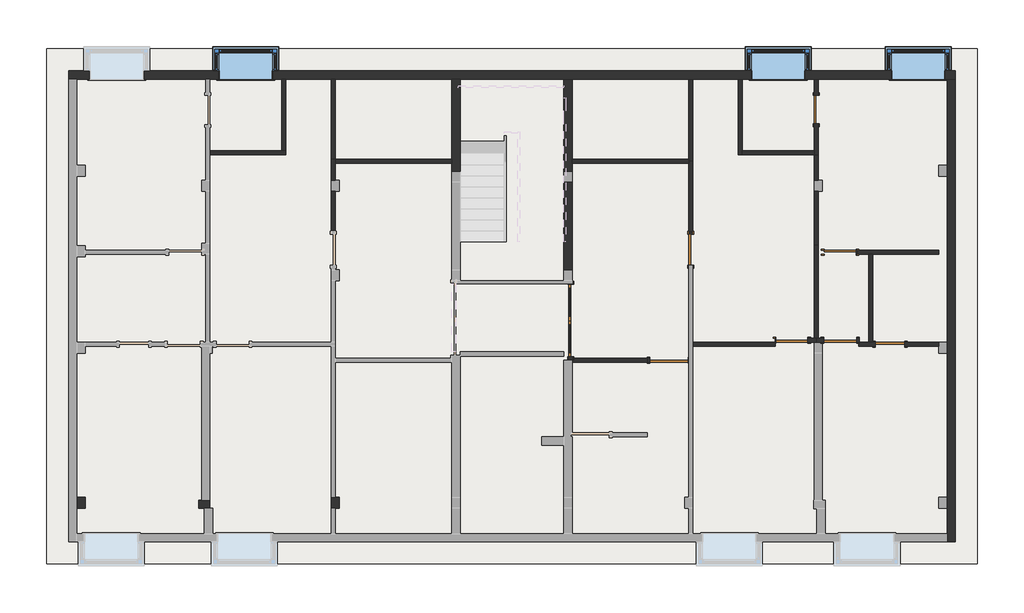
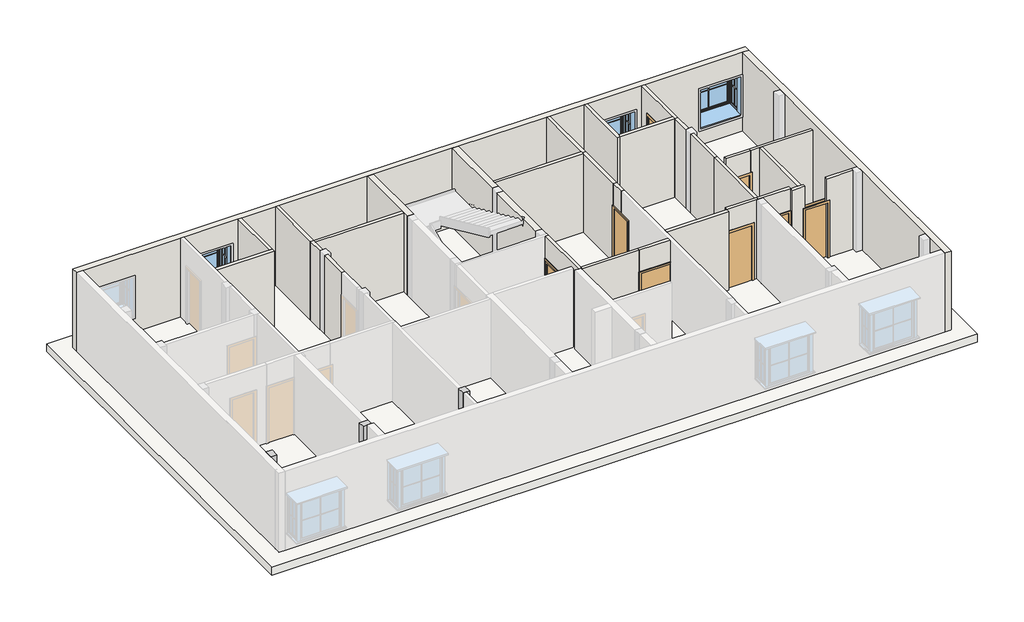
# One storey, part 2 of 3: 32 walls, 8 doors, 3 columns, 3 windows, 1 slab.
"""IFC4 building model written with IfcOpenShell, lengths in millimetres."""

from ifc_helpers import new_model, si_unit, frame, origin, place, context, project, spatial, polyline, outline, extrude, faceted_brep, transform, mapped, element, save
from components import door_04ab2522, m_door_single_panel_05506f71, door_85b31ab1, door_1991e9a2, door_a431d384, door_82def9da, m_door_single_panel_3_x7_f8176753, window_19bbd869

model = new_model("IFC4")

# Units and contexts
model_context = context("Model", 3, world=origin())
ifc_project = project(units=[si_unit("LENGTHUNIT", "METRE", prefix="MILLI")], contexts=[model_context])

# Site, building, storey
site = spatial("IfcSite", under=ifc_project)
building = spatial("IfcBuilding", under=site)
storey = spatial("IfcBuildingStorey", under=building, Elevation=6400.8)

# Columns
placement = place(None, origin())
element("IfcColumn", 1, ObjectType="Rectangular Column : 1'X 9\"", at=placement, inside=storey, context=model_context, shape_type="SweptSolid", body=[
    extrude(outline(polyline([(-12224.6987957, -3709.2932671), (-12224.6987957, -4014.0932671), (-12453.2987957, -4014.0932671), (-12453.2987957, -3709.2932671), (-12224.6987957, -3709.2932671)])), frame((0.0, 0.0, 6400.8), z_axis=(0.0, 0.0, 1.0), x_axis=(1.0, 0.0, 0.0)), (0.0, 0.0, 1.0), 3048.0),
])
element("IfcColumn", 2, ObjectType="Rectangular Column : 1'X 9\"", at=placement, inside=storey, context=model_context, shape_type="Brep", body=[
    faceted_brep([(-5188.8987963, -3709.2932193, 6400.8), (-5188.8987963, -4014.0932193, 6400.8), (-5303.1987963, -4014.0932193, 6400.8), (-5417.4987963, -4014.0932193, 6400.8), (-5417.4987963, -3709.2932193, 6400.8), (-5303.1987995, -3709.2932193, 6400.8), (-5188.8987963, -3709.2932193, 9448.8), (-5188.8987963, -4014.0932193, 9448.8), (-5303.1987963, -4014.0932193, 9448.8), (-5417.4987963, -4014.0932193, 9448.8), (-5417.4987963, -3709.2932193, 9448.8), (-5303.1987995, -3709.2932193, 9448.8)], [[[0, 1, 2, 3, 4, 5]], [[6, 7, 1, 0]], [[7, 8, 9, 3, 2, 1]], [[9, 10, 4, 3]], [[10, 11, 6, 0, 5, 4]], [[6, 11, 10, 9, 8, 7]]]),
])
element("IfcColumn", 3, ObjectType="Rectangular Column : 1'X 9\"", at=placement, inside=storey, context=model_context, shape_type="Brep", body=[
    faceted_brep([(-9076.550543, -3785.4932196, 6400.8), (-9000.350543, -3785.4932196, 6400.8), (-8771.750543, -3785.4932196, 6400.8), (-8771.750543, -4014.0932196, 6400.8), (-8924.150543, -4014.0932196, 6400.8), (-9076.550543, -4014.0932196, 6400.8), (-9076.550543, -3785.4932196, 9448.8), (-9000.350543, -3785.4932196, 9448.8), (-8771.750543, -3785.4932196, 9448.8), (-8771.750543, -4014.0932196, 9448.8), (-8924.150543, -4014.0932196, 9448.8), (-9076.550543, -4014.0932196, 9448.8)], [[[0, 1, 2, 3, 4, 5]], [[6, 7, 8, 2, 1, 0]], [[8, 9, 3, 2]], [[9, 10, 11, 5, 4, 3]], [[11, 6, 0, 5]], [[6, 11, 10, 9, 8, 7]]]),
])

# Doors
door_shape = door_04ab2522(model_context)
element("IfcDoor", 4, ObjectType="M_Door-Double-Glass : 6'7\"X7'", at=placement, inside=storey, context=model_context, shape_type="MappedRepresentation", body=[
    mapped(door_shape, transform((1217.5394962, 1183.3817656, 6400.8), x_axis=(0.0, 1.0, 0.0), y_axis=(-1.0, 0.0, 0.0), z_axis=(0.0, 0.0, 1.0))),
])
m_door_single_panel_shape = m_door_single_panel_05506f71(model_context)
element("IfcDoor", 5, ObjectType="M_Door-Single-Panel", at=placement, inside=storey, context=model_context, shape_type="MappedRepresentation", body=[
    mapped(m_door_single_panel_shape, transform((3933.4813133, 90.9578621, 6400.8), x_axis=(1.0, 0.0, 0.0), y_axis=(0.0, 1.0, 0.0), z_axis=(0.0, 0.0, 1.0))),
])
door_2_shape = door_85b31ab1(model_context)
element("IfcDoor", 6, ObjectType="M_Door-Single-Panel : 2'10\"X7' 2", at=placement, inside=storey, context=model_context, shape_type="MappedRepresentation", body=[
    mapped(door_2_shape, transform((4532.9512082, 3142.9626891, 6400.8), x_axis=(0.0, -1.0, 0.0), y_axis=(1.0, 0.0, 0.0), z_axis=(0.0, 0.0, 1.0))),
])
door_3_shape = door_1991e9a2(model_context)
element("IfcDoor", 7, ObjectType="M_Door-Single-Panel : 2'11\"X7' 3", at=placement, inside=storey, context=model_context, shape_type="MappedRepresentation", body=[
    mapped(door_3_shape, transform((7330.1405552, 640.4567334, 6400.8), x_axis=(1.0, 0.0, 0.0), y_axis=(0.0, 1.0, 0.0), z_axis=(0.0, 0.0, 1.0))),
])
element("IfcDoor", 8, ObjectType="M_Door-Single-Panel : 2'11\"X7' 3", at=placement, inside=storey, context=model_context, shape_type="MappedRepresentation", body=[
    mapped(door_3_shape, transform((8664.274939, 3078.8567332, 6400.8), x_axis=(-1.0, 0.0, 0.0), y_axis=(0.0, -1.0, 0.0), z_axis=(0.0, 0.0, 1.0))),
])
door_4_shape = door_a431d384(model_context)
element("IfcDoor", 9, ObjectType="M_Door-Single-Panel : 2'7\"X7' 2", at=placement, inside=storey, context=model_context, shape_type="MappedRepresentation", body=[
    mapped(door_4_shape, transform((8000.0512079, 7021.3751452, 6400.8), x_axis=(0.0, 1.0, 0.0), y_axis=(-1.0, 0.0, 0.0), z_axis=(0.0, 0.0, 1.0))),
])
door_5_shape = door_82def9da(model_context)
element("IfcDoor", 10, ObjectType="M_Door-Single-Panel : 2'8\"X7'", at=placement, inside=storey, context=model_context, shape_type="MappedRepresentation", body=[
    mapped(door_5_shape, transform((10046.0486694, 526.1567295, 6400.8), x_axis=(-1.0, 0.0, 0.0), y_axis=(0.0, -1.0, 0.0), z_axis=(0.0, 0.0, 1.0))),
])
m_door_single_panel_3_x7_shape = m_door_single_panel_3_x7_f8176753(model_context)
element("IfcDoor", 11, ObjectType="M_Door-Single-Panel : 3'X7'", at=placement, inside=storey, context=model_context, shape_type="MappedRepresentation", body=[
    mapped(m_door_single_panel_3_x7_shape, transform((8666.8012079, 640.4567334, 6400.8), x_axis=(-1.0, 0.0, 0.0), y_axis=(0.0, -1.0, 0.0), z_axis=(0.0, 0.0, 1.0))),
])

# Slab
element("IfcSlab", 12, ObjectType="Generic - 12\"", at=placement, inside=storey, context=model_context, shape_type="SweptSolid", body=[
    extrude(outline(polyline([(12464.1012075, 8698.6067329), (12464.1012075, -5550.7932662), (-13291.4987957, -5550.7932662), (-13291.4987957, 8698.6067329), (12464.1012075, 8698.6067329)])), frame((0.0, 0.0, 6096.0), z_axis=(0.0, 0.0, 1.0), x_axis=(1.0, 0.0, 0.0)), (0.0, 0.0, 1.0), 304.8),
])

# Walls
element("IfcWall", 13, ObjectType="4.5\"", at=placement, inside=storey, context=model_context, shape_type="SweptSolid", body=[
    extrude(outline(polyline([(3132.0737955, 9448.8), (3628.3344162, 9448.8), (3628.3344162, 6400.8), (3574.7626891, 6400.8), (3574.7626891, 8534.4), (3132.0737955, 8534.4), (3132.0737955, 9448.8)])), frame((4475.8012082, 0.0, 0.0), z_axis=(1.0, 0.0, 0.0), x_axis=(0.0, 1.0, 0.0)), (0.0, 0.0, 1.0), 114.3),
])
element("IfcWall", 14, ObjectType="4.5\"", at=placement, inside=storey, context=model_context, shape_type="Brep", body=[
    faceted_brep([(8000.0512079, 583.3067334, 6400.8), (8000.0512079, 583.3067334, 9448.8), (7942.9012047, 583.3067334, 9448.8), (6862.7668241, 583.3067334, 9448.8), (6862.7668241, 583.3067334, 6400.8), (6885.6405552, 583.3067334, 6400.8), (6885.6405552, 583.3067334, 8534.4), (7774.6405552, 583.3067334, 8534.4), (7774.6405552, 583.3067334, 6400.8), (7942.9012047, 583.3067334, 6400.8), (8000.0512079, 697.6067334, 9448.8), (8000.0512079, 697.6067334, 6400.8), (7942.9012079, 697.6067334, 6400.8), (7774.6405552, 697.6067334, 6400.8), (7774.6405552, 697.6067334, 8534.4), (6885.6405552, 697.6067334, 8534.4), (6885.6405552, 697.6067334, 6400.8), (6862.7668241, 697.6067334, 6400.8), (6862.7668241, 697.6067334, 9448.8), (7942.9012079, 697.6067334, 9448.8)], [[[0, 1, 2, 3, 4, 5, 6, 7, 8, 9]], [[10, 11, 12, 13, 14, 15, 16, 17, 18, 19]], [[4, 17, 16, 5]], [[11, 0, 9, 8, 13, 12]], [[1, 0, 11, 10]], [[3, 2, 1, 10, 19, 18]], [[4, 3, 18, 17]], [[7, 14, 13, 8]], [[14, 7, 6, 15]], [[15, 6, 5, 16]]]),
])
element("IfcWall", 15, ObjectType="4.5\"", at=placement, inside=storey, context=model_context, shape_type="Brep", body=[
    faceted_brep([(9187.5012047, 583.3067334, 6400.8), (9187.5012047, 583.3067334, 9448.8), (8171.5012047, 583.3067334, 9448.8), (8000.0512079, 583.3067334, 9448.8), (8000.0512079, 583.3067334, 6400.8), (8171.5012047, 583.3067334, 6400.8), (8209.6012079, 583.3067334, 6400.8), (8209.6012079, 583.3067334, 8534.4), (9124.0012079, 583.3067334, 8534.4), (9124.0012079, 583.3067334, 6400.8), (9187.5012047, 697.6067334, 9448.8), (9187.5012047, 697.6067334, 6400.8), (9124.0012079, 697.6067334, 6400.8), (9124.0012079, 697.6067334, 8534.4), (8209.6012079, 697.6067334, 8534.4), (8209.6012079, 697.6067334, 6400.8), (8057.2012079, 697.6067334, 6400.8), (8000.0512079, 697.6067334, 6400.8), (8000.0512079, 697.6067334, 9448.8), (8057.2012079, 697.6067334, 9448.8)], [[[0, 1, 2, 3, 4, 5, 6, 7, 8, 9]], [[10, 11, 12, 13, 14, 15, 16, 17, 18, 19]], [[11, 0, 9, 12]], [[4, 17, 16, 15, 6, 5]], [[1, 0, 11, 10]], [[3, 2, 1, 10, 19, 18]], [[4, 3, 18, 17]], [[7, 14, 13, 8]], [[8, 13, 12, 9]], [[14, 7, 6, 15]]]),
])
element("IfcWall", 16, ObjectType="4.5\"", at=placement, inside=storey, context=model_context, shape_type="SweptSolid", body=[
    extrude(outline(polyline([(6400.8, 9131.6486701), (9448.8, 9131.6486701), (9448.8, 8245.174939), (8534.4, 8245.174939), (8534.4, 9108.774939), (6400.8, 9108.774939), (6400.8, 9131.6486701)])), frame((0.0, 3021.7067332, 0.0), z_axis=(0.0, 1.0, 0.0), x_axis=(0.0, 0.0, 1.0)), (0.0, 0.0, 1.0), 114.3),
])
element("IfcWall", 17, ObjectType="4.5\"", at=placement, inside=storey, context=model_context, shape_type="Brep", body=[
    faceted_brep([(7942.9012079, 5764.9067329, 9448.8), (7942.9012079, 5879.2067329, 9448.8), (7942.9012079, 7860.4067329, 9448.8), (7942.9012079, 7860.4067329, 6400.8), (7942.9012079, 7415.0751452, 6400.8), (7942.9012079, 7415.0751452, 8534.4), (7942.9012079, 6627.6751452, 8534.4), (7942.9012079, 6627.6751452, 6400.8), (7942.9012079, 5879.2067329, 6400.8), (7942.9012079, 5764.9067329, 6400.8), (8057.2012079, 7860.4067329, 9448.8), (8057.2012079, 5764.9067329, 9448.8), (8057.2012079, 5764.9067329, 6400.8), (8057.2012079, 6627.6751452, 6400.8), (8057.2012079, 6627.6751452, 8534.4), (8057.2012079, 7415.0751452, 8534.4), (8057.2012079, 7415.0751452, 6400.8), (8057.2012079, 7860.4067329, 6400.8)], [[[0, 1, 2, 3, 4, 5, 6, 7, 8, 9]], [[10, 11, 12, 13, 14, 15, 16, 17]], [[12, 9, 8, 7, 13]], [[3, 17, 16, 4]], [[2, 1, 0, 11, 10]], [[15, 5, 4, 16]], [[5, 15, 14, 6]], [[6, 14, 13, 7]], [[0, 9, 12, 11]], [[3, 2, 10, 17]]]),
])
element("IfcWall", 18, ObjectType="4.5\"", at=placement, inside=storey, context=model_context, shape_type="SweptSolid", body=[
    extrude(outline(polyline([(8534.4, 4466.8813133), (6400.8, 4466.8813133), (6400.8, 4475.8012082), (9448.8, 4475.8012082), (9448.8, 3334.0114184), (6400.8, 3334.0114184), (6400.8, 3400.0813133), (8534.4, 3400.0813133), (8534.4, 4466.8813133)])), frame((0.0, 33.8078621, 0.0), z_axis=(0.0, 1.0, 0.0), x_axis=(0.0, 0.0, 1.0)), (0.0, 0.0, 1.0), 114.3),
])
element("IfcWall", 19, ObjectType="4.5\"", at=placement, inside=storey, context=model_context, shape_type="Brep", body=[
    faceted_brep([(1158.0082462, 2196.2067742, 6400.8), (1158.0082462, 2186.6817656, 6400.8), (1158.0082462, 2186.6817656, 8534.4), (1158.0082462, 180.0817656, 8534.4), (1158.0082462, 180.0817656, 6400.8), (1158.0082462, 90.9578621, 6400.8), (1158.0082462, 90.9578621, 9448.8), (1158.0082462, 2196.2067742, 9448.8), (1272.3082462, 2186.6817656, 8534.4), (1272.3082462, 2186.6817656, 6400.8), (1272.3082462, 2196.2067742, 6400.8), (1272.3082462, 2196.2067742, 9448.8), (1272.3082462, 148.1078621, 9448.8), (1272.3082462, 90.9578621, 9448.8), (1272.3082462, 90.9578621, 6400.8), (1272.3082462, 148.1078621, 6400.8), (1272.3082462, 180.0817656, 6400.8), (1272.3082462, 180.0817656, 8534.4), (1250.0012085, 90.9578621, 6400.8), (1250.0012085, 90.9578621, 9448.8)], [[[0, 1, 2, 3, 4, 5, 6, 7]], [[8, 9, 10, 11, 12, 13, 14, 15, 16, 17]], [[10, 9, 1, 0]], [[16, 15, 14, 18, 5, 4]], [[6, 5, 18, 14, 13, 19]], [[7, 6, 19, 13, 12, 11]], [[0, 7, 11, 10]], [[2, 1, 9, 8]], [[3, 2, 8, 17]], [[4, 3, 17, 16]]]),
])
element("IfcWall", 20, ObjectType="4.5\"", at=placement, inside=storey, context=model_context, shape_type="Brep", body=[
    faceted_brep([(1250.0012085, 5536.3067329, 6400.8), (4475.8012082, 5536.3067329, 6400.8), (4475.8012082, 5536.3067329, 9448.8), (1250.0012085, 5536.3067329, 9448.8), (1250.0012085, 5650.6067329, 6400.8), (1250.0012085, 5650.6067329, 9448.8), (4475.8012082, 5650.6067329, 9448.8), (4475.8012082, 5650.6067329, 6400.8), (4475.8012082, 5593.4567329, 6400.8), (4475.8012082, 5593.4567329, 9448.8)], [[[0, 1, 2, 3]], [[4, 5, 6, 7]], [[1, 0, 4, 7, 8]], [[3, 2, 9, 6, 5]], [[2, 1, 8, 7, 6, 9]], [[0, 3, 5, 4]]]),
])
element("IfcWall", 21, ObjectType="4.5\"", at=placement, inside=storey, context=model_context, shape_type="Brep", body=[
    faceted_brep([(8057.2012047, 3270.1432417, 6400.8), (8057.2012047, 4760.6824989, 6400.8), (8057.2012047, 4760.6824989, 9448.8), (8057.2012047, 3270.1432417, 9448.8), (7942.9012047, 3270.1432417, 6400.8), (7942.9012047, 3270.1432417, 9448.8), (7942.9012047, 4760.6824989, 9448.8), (7942.9012047, 4760.6824989, 6400.8), (7943.9040565, 4760.6824989, 6400.8), (7943.9040565, 4760.6824989, 9448.8)], [[[0, 1, 2, 3]], [[4, 5, 6, 7]], [[1, 0, 4, 7, 8]], [[2, 1, 8, 7, 6, 9]], [[3, 2, 9, 6, 5]], [[0, 3, 5, 4]]]),
])
element("IfcWall", 22, ObjectType="4.5\"", at=placement, inside=storey, context=model_context, shape_type="Brep", body=[
    faceted_brep([(7942.9012079, 3270.1432417, 6400.8), (7942.9012079, 697.6067334, 6400.8), (7942.9012079, 697.6067334, 9448.8), (7942.9012079, 3270.1432417, 9448.8), (8057.2012079, 3270.1432417, 6400.8), (8057.2012079, 3270.1432417, 9448.8), (8057.2012079, 697.6067334, 9448.8), (8057.2012079, 697.6067334, 6400.8), (8000.0512079, 697.6067334, 6400.8), (8000.0512079, 697.6067334, 9448.8)], [[[0, 1, 2, 3]], [[4, 5, 6, 7]], [[1, 0, 4, 7, 8]], [[3, 2, 9, 6, 5]], [[0, 3, 5, 4]], [[2, 1, 8, 7, 6, 9]]]),
])
element("IfcWall", 23, ObjectType="4.5\"", at=placement, inside=storey, context=model_context, shape_type="SweptSolid", body=[
    extrude(outline(polyline([(8058.2040565, 5763.9824989), (8058.2040565, 5065.4824989), (7943.9040565, 5065.4824989), (7943.9040565, 5763.9824989), (8058.2040565, 5763.9824989)])), frame((0.0, 0.0, 6400.8), z_axis=(0.0, 0.0, 1.0), x_axis=(1.0, 0.0, 0.0)), (0.0, 0.0, 1.0), 3048.0),
])
element("IfcWall", 24, ObjectType="4.5\"", at=placement, inside=storey, context=model_context, shape_type="SweptSolid", body=[
    extrude(outline(polyline([(1272.3082462, 148.1078621), (3334.0114184, 148.1078621), (3334.0114184, 33.8078621), (1250.0012085, 33.8078621), (1250.0012085, 90.9578621), (1272.3082462, 90.9578621), (1272.3082462, 148.1078621)])), frame((0.0, 0.0, 6400.8), z_axis=(0.0, 0.0, 1.0), x_axis=(1.0, 0.0, 0.0)), (0.0, 0.0, 1.0), 3048.0),
])
element("IfcWall", 25, ObjectType="4.5\" 2", at=placement, inside=storey, context=model_context, shape_type="Brep", body=[
    faceted_brep([(-8770.2987992, 5764.9067329, 6400.8), (-6674.7987994, 5764.9067329, 6400.8), (-6674.7987994, 5764.9067329, 9448.8), (-8770.2987992, 5764.9067329, 9448.8), (-8770.2987992, 5879.2067329, 6400.8), (-8770.2987992, 5879.2067329, 9448.8), (-6789.0987994, 5879.2067329, 9448.8), (-6674.7987994, 5879.2067329, 9448.8), (-6674.7987994, 5879.2067329, 6400.8), (-6789.0987994, 5879.2067329, 6400.8)], [[[0, 1, 2, 3]], [[4, 5, 6, 7, 8, 9]], [[1, 0, 4, 9, 8]], [[3, 2, 7, 6, 5]], [[0, 3, 5, 4]], [[2, 1, 8, 7]]]),
])
element("IfcWall", 26, ObjectType="4.5\" 2", at=placement, inside=storey, context=model_context, shape_type="SweptSolid", body=[
    extrude(outline(polyline([(-6674.7987994, 7860.4067329), (-6674.7987994, 5879.2067329), (-6789.0987994, 5879.2067329), (-6789.0987994, 7860.4067329), (-6674.7987994, 7860.4067329)])), frame((0.0, 0.0, 6400.8), z_axis=(0.0, 0.0, 1.0), x_axis=(1.0, 0.0, 0.0)), (0.0, 0.0, 1.0), 3048.0),
])
element("IfcWall", 27, ObjectType="4.5\" 2", at=placement, inside=storey, context=model_context, shape_type="SweptSolid", body=[
    extrude(outline(polyline([(-5303.1987995, 4761.606733), (-5303.1987995, 3671.8272228), (-5417.4987995, 3671.8272228), (-5417.4987995, 4761.606733), (-5303.1987995, 4761.606733)])), frame((0.0, 0.0, 6400.8), z_axis=(0.0, 0.0, 1.0), x_axis=(1.0, 0.0, 0.0)), (0.0, 0.0, 1.0), 3048.0),
])
element("IfcWall", 28, ObjectType="4.5\" 2", at=placement, inside=storey, context=model_context, shape_type="Brep", body=[
    faceted_brep([(-5303.1987995, 5066.406733, 6400.8), (-5303.1987995, 5536.3067329, 6400.8), (-5303.1987995, 5650.6067329, 6400.8), (-5303.1987995, 5650.6067329, 9448.8), (-5303.1987995, 5536.3067329, 9448.8), (-5303.1987995, 5066.406733, 9448.8), (-5417.4987995, 5066.406733, 6400.8), (-5417.4987995, 5066.406733, 9448.8), (-5417.4987995, 5650.6067329, 9448.8), (-5417.4987995, 5650.6067329, 6400.8)], [[[0, 1, 2, 3, 4, 5]], [[6, 7, 8, 9]], [[2, 1, 0, 6, 9]], [[5, 4, 3, 8, 7]], [[0, 5, 7, 6]], [[3, 2, 9, 8]]]),
])
element("IfcWall", 29, ObjectType="4.5\" 2", at=placement, inside=storey, context=model_context, shape_type="SweptSolid", body=[
    extrude(outline(polyline([(-2077.3987998, 5536.3067329), (-5303.1987995, 5536.3067329), (-5303.1987995, 5650.6067329), (-2077.3987998, 5650.6067329), (-2077.3987998, 5536.3067329)])), frame((0.0, 0.0, 6400.8), z_axis=(0.0, 0.0, 1.0), x_axis=(1.0, 0.0, 0.0)), (0.0, 0.0, 1.0), 3048.0),
])
element("IfcWall", 30, ObjectType="4.5\" 2", at=placement, inside=storey, context=model_context, shape_type="SweptSolid", body=[
    extrude(outline(polyline([(-5417.4987995, 5650.6067329), (-5417.4987995, 7860.4067329), (-5303.1987995, 7860.4067329), (-5303.1987995, 5650.6067329), (-5417.4987995, 5650.6067329)])), frame((0.0, 0.0, 6400.8), z_axis=(0.0, 0.0, 1.0), x_axis=(1.0, 0.0, 0.0)), (0.0, 0.0, 1.0), 3048.0),
])
element("IfcWall", 31, ObjectType="4.5\" 2", at=placement, inside=storey, context=model_context, shape_type="Brep", body=[
    faceted_brep([(4475.8012082, 5593.4567329, 6400.8), (4475.8012082, 5536.3067329, 6400.8), (4475.8012082, 3628.3344162, 6400.8), (4475.8012082, 3628.3344162, 9448.8), (4475.8012082, 5536.3067329, 9448.8), (4475.8012082, 5593.4567329, 9448.8), (4590.1012082, 5593.4567329, 6400.8), (4590.1012082, 5593.4567329, 9448.8), (4590.1012082, 3628.3344162, 9448.8), (4590.1012082, 3628.3344162, 6400.8)], [[[0, 1, 2, 3, 4, 5]], [[6, 7, 8, 9]], [[2, 1, 0, 6, 9]], [[3, 2, 9, 8]], [[5, 4, 3, 8, 7]], [[0, 5, 7, 6]]]),
])
element("IfcWall", 32, ObjectType="4.5\" 2", at=placement, inside=storey, context=model_context, shape_type="SweptSolid", body=[
    extrude(outline(polyline([(6862.7668241, 469.0067334), (4590.1012082, 469.0067334), (4590.1012082, 583.3067334), (6862.7668241, 583.3067334), (6862.7668241, 469.0067334)])), frame((0.0, 0.0, 6400.8), z_axis=(0.0, 0.0, 1.0), x_axis=(1.0, 0.0, 0.0)), (0.0, 0.0, 1.0), 3048.0),
])
element("IfcWall", 33, ObjectType="4.5\" 2", at=placement, inside=storey, context=model_context, shape_type="Brep", body=[
    faceted_brep([(9182.4486694, 469.0067295, 6400.8), (9639.6486694, 469.0067295, 6400.8), (9639.6486694, 469.0067295, 9448.8), (9182.4486694, 469.0067295, 9448.8), (9182.4486694, 583.3067295, 6400.8), (9182.4486694, 583.3067295, 9448.8), (9451.1098918, 583.3067295, 9448.8), (9565.4098918, 583.3067295, 9448.8), (9639.6486694, 583.3067295, 9448.8), (9639.6486694, 583.3067295, 6400.8), (9565.4098918, 583.3067295, 6400.8), (9451.1098918, 583.3067295, 6400.8)], [[[0, 1, 2, 3]], [[4, 5, 6, 7, 8, 9, 10, 11]], [[1, 0, 4, 11, 10, 9]], [[2, 1, 9, 8]], [[3, 2, 8, 7, 6, 5]], [[0, 3, 5, 4]]]),
])
element("IfcWall", 34, ObjectType="4.5\" 2", at=placement, inside=storey, context=model_context, shape_type="SweptSolid", body=[
    extrude(outline(polyline([(6400.8, 11397.3012075), (9448.8, 11397.3012075), (9448.8, 10443.8236977), (8534.4, 10443.8236977), (8534.4, 10452.4486694), (6400.8, 10452.4486694), (6400.8, 11397.3012075)])), frame((0.0, 469.0067295, 0.0), z_axis=(0.0, 1.0, 0.0), x_axis=(0.0, 0.0, 1.0)), (0.0, 0.0, 1.0), 114.3),
])
element("IfcWall", 35, ObjectType="4.5\" 2", at=placement, inside=storey, context=model_context, shape_type="SweptSolid", body=[
    extrude(outline(polyline([(9565.4098918, 3021.7067332), (9565.4098918, 583.3067295), (9451.1098918, 583.3067295), (9451.1098918, 3021.7067332), (9565.4098918, 3021.7067332)])), frame((0.0, 0.0, 6400.8), z_axis=(0.0, 0.0, 1.0), x_axis=(1.0, 0.0, 0.0)), (0.0, 0.0, 1.0), 3048.0),
])
element("IfcWall", 36, ObjectType="4.5\" 2", at=placement, inside=storey, context=model_context, shape_type="Brep", body=[
    faceted_brep([(9131.6486701, 3021.7067332, 6400.8), (9451.1098918, 3021.7067332, 6400.8), (9565.4098918, 3021.7067332, 6400.8), (11397.3012075, 3021.7067332, 6400.8), (11397.3012075, 3021.7067332, 9448.8), (9565.4098918, 3021.7067332, 9448.8), (9451.1098918, 3021.7067332, 9448.8), (9131.6486701, 3021.7067332, 9448.8), (9131.6486701, 3136.0067332, 6400.8), (9131.6486701, 3136.0067332, 9448.8), (11397.3012075, 3136.0067332, 9448.8), (11397.3012075, 3136.0067332, 6400.8)], [[[0, 1, 2, 3, 4, 5, 6, 7]], [[8, 9, 10, 11]], [[3, 2, 1, 0, 8, 11]], [[4, 3, 11, 10]], [[7, 6, 5, 4, 10, 9]], [[0, 7, 9, 8]]]),
])
element("IfcWall", 37, ObjectType="4.5\" 2", at=placement, inside=storey, context=model_context, shape_type="Brep", body=[
    faceted_brep([(4590.1012082, 5593.4567329, 6400.8), (4590.1012082, 7860.4067329, 6400.8), (4590.1012082, 7860.4067329, 9448.8), (4590.1012082, 5593.4567329, 9448.8), (4475.8012082, 5593.4567329, 6400.8), (4475.8012082, 5593.4567329, 9448.8), (4475.8012082, 5650.6067329, 9448.8), (4475.8012082, 7860.4067329, 9448.8), (4475.8012082, 7860.4067329, 6400.8), (4475.8012082, 5650.6067329, 6400.8)], [[[0, 1, 2, 3]], [[4, 5, 6, 7, 8, 9]], [[1, 0, 4, 9, 8]], [[3, 2, 7, 6, 5]], [[0, 3, 5, 4]], [[2, 1, 8, 7]]]),
])
element("IfcWall", 38, ObjectType="4.5\" 2", at=placement, inside=storey, context=model_context, shape_type="Brep", body=[
    faceted_brep([(5847.401208, 7860.4067329, 6400.8), (5847.401208, 5764.9067329, 6400.8), (5847.401208, 5764.9067329, 9448.8), (5847.401208, 7860.4067329, 9448.8), (5961.701208, 7860.4067329, 6400.8), (5961.701208, 7860.4067329, 9448.8), (5961.701208, 5879.2067329, 9448.8), (5961.701208, 5764.9067329, 9448.8), (5961.701208, 5764.9067329, 6400.8), (5961.701208, 5879.2067329, 6400.8)], [[[0, 1, 2, 3]], [[4, 5, 6, 7, 8, 9]], [[1, 0, 4, 9, 8]], [[3, 2, 7, 6, 5]], [[2, 1, 8, 7]], [[0, 3, 5, 4]]]),
])
element("IfcWall", 39, ObjectType="4.5\" 2", at=placement, inside=storey, context=model_context, shape_type="SweptSolid", body=[
    extrude(outline(polyline([(7942.9012079, 5764.9067329), (5961.701208, 5764.9067329), (5961.701208, 5879.2067329), (7942.9012079, 5879.2067329), (7942.9012079, 5764.9067329)])), frame((0.0, 0.0, 6400.8), z_axis=(0.0, 0.0, 1.0), x_axis=(1.0, 0.0, 0.0)), (0.0, 0.0, 1.0), 3048.0),
])
element("IfcWall", 40, ObjectType="9\"", at=placement, inside=storey, context=model_context, shape_type="Brep", body=[
    faceted_brep([(-12681.8987957, 7860.4067329, 6400.8), (-12453.2987957, 7860.4067329, 6400.8), (-8884.5987992, 7860.4067329, 6400.8), (-8770.2987992, 7860.4067329, 6400.8), (-6789.0987994, 7860.4067329, 6400.8), (-6674.7987994, 7860.4067329, 6400.8), (-5417.4987995, 7860.4067329, 6400.8), (-5303.1987995, 7860.4067329, 6400.8), (-2074.1417538, 7860.4067329, 6400.8), (-1845.5417538, 7860.4067329, 6400.8), (1021.4012085, 7860.4067329, 6400.8), (1250.0012085, 7860.4067329, 6400.8), (4475.8012082, 7860.4067329, 6400.8), (4590.1012082, 7860.4067329, 6400.8), (5847.401208, 7860.4067329, 6400.8), (5961.701208, 7860.4067329, 6400.8), (7942.9012079, 7860.4067329, 6400.8), (8057.2012079, 7860.4067329, 6400.8), (11625.9012075, 7860.4067329, 6400.8), (11854.5012075, 7860.4067329, 6400.8), (11854.5012075, 7860.4067329, 9448.8), (11625.9012075, 7860.4067329, 9448.8), (8057.2012079, 7860.4067329, 9448.8), (7942.9012079, 7860.4067329, 9448.8), (5961.701208, 7860.4067329, 9448.8), (5847.401208, 7860.4067329, 9448.8), (4590.1012082, 7860.4067329, 9448.8), (4475.8012082, 7860.4067329, 9448.8), (1250.0012085, 7860.4067329, 9448.8), (1021.4012085, 7860.4067329, 9448.8), (-1845.5417538, 7860.4067329, 9448.8), (-2074.1417538, 7860.4067329, 9448.8), (-5303.1987995, 7860.4067329, 9448.8), (-5417.4987995, 7860.4067329, 9448.8), (-6674.7987994, 7860.4067329, 9448.8), (-6789.0987994, 7860.4067329, 9448.8), (-8770.2987992, 7860.4067329, 9448.8), (-8884.5987992, 7860.4067329, 9448.8), (-12453.2987957, 7860.4067329, 9448.8), (-12681.8987957, 7860.4067329, 9448.8), (11575.8012075, 7860.4067329, 8551.6), (11575.8012075, 7860.4067329, 7000.8), (10075.8012075, 7860.4067329, 7000.8), (10075.8012075, 7860.4067329, 8551.6), (7702.301208, 7860.4067329, 8551.6), (7702.301208, 7860.4067329, 7000.8), (6202.301208, 7860.4067329, 7000.8), (6202.301208, 7860.4067329, 8551.6), (-7029.6987993, 7860.4067329, 8551.6), (-7029.6987993, 7860.4067329, 7000.8), (-8529.6987993, 7860.4067329, 7000.8), (-8529.6987993, 7860.4067329, 8551.6), (-10598.3987957, 7860.4067329, 8551.6), (-10598.3987957, 7860.4067329, 7000.8), (-12098.3987957, 7860.4067329, 7000.8), (-12098.3987957, 7860.4067329, 8551.6), (-12681.8987957, 8089.0067329, 6400.8), (-12681.8987957, 8089.0067329, 9448.8), (11854.5012075, 8089.0067329, 9448.8), (11854.5012075, 8089.0067329, 6400.8), (11575.8012075, 8089.0067329, 8551.6), (10075.8012075, 8089.0067329, 8551.6), (10075.8012075, 8089.0067329, 7000.8), (11575.8012075, 8089.0067329, 7000.8), (7702.301208, 8089.0067329, 8551.6), (6202.301208, 8089.0067329, 8551.6), (6202.301208, 8089.0067329, 7000.8), (7702.301208, 8089.0067329, 7000.8), (-7029.6987993, 8089.0067329, 8551.6), (-8529.6987993, 8089.0067329, 8551.6), (-8529.6987993, 8089.0067329, 7000.8), (-7029.6987993, 8089.0067329, 7000.8), (-10598.3987957, 8089.0067329, 8551.6), (-12098.3987957, 8089.0067329, 8551.6), (-12098.3987957, 8089.0067329, 7000.8), (-10598.3987957, 8089.0067329, 7000.8)], [[[0, 1, 2, 3, 4, 5, 6, 7, 8, 9, 10, 11, 12, 13, 14, 15, 16, 17, 18, 19, 20, 21, 22, 23, 24, 25, 26, 27, 28, 29, 30, 31, 32, 33, 34, 35, 36, 37, 38, 39], [40, 41, 42, 43], [44, 45, 46, 47], [48, 49, 50, 51], [52, 53, 54, 55]], [[56, 57, 58, 59], [60, 61, 62, 63], [64, 65, 66, 67], [68, 69, 70, 71], [72, 73, 74, 75]], [[19, 18, 17, 16, 15, 14, 13, 12, 11, 10, 9, 8, 7, 6, 5, 4, 3, 2, 1, 0, 56, 59]], [[39, 38, 37, 36, 35, 34, 33, 32, 31, 30, 29, 28, 27, 26, 25, 24, 23, 22, 21, 20, 58, 57]], [[20, 19, 59, 58]], [[0, 39, 57, 56]], [[41, 40, 60, 63]], [[42, 41, 63, 62]], [[43, 42, 62, 61]], [[40, 43, 61, 60]], [[45, 44, 64, 67]], [[46, 45, 67, 66]], [[47, 46, 66, 65]], [[44, 47, 65, 64]], [[49, 48, 68, 71]], [[50, 49, 71, 70]], [[51, 50, 70, 69]], [[48, 51, 69, 68]], [[53, 52, 72, 75]], [[54, 53, 75, 74]], [[55, 54, 74, 73]], [[52, 55, 73, 72]]]),
])
element("IfcWall", 41, ObjectType="9\"", at=placement, inside=storey, context=model_context, shape_type="Brep", body=[
    faceted_brep([(11625.9012075, 7860.4067329, 6400.8), (11625.9012075, 5479.1567329, 6400.8), (11625.9012075, 5174.3567329, 6400.8), (11625.9012075, 583.3067295, 6400.8), (11625.9012075, 278.5067295, 6400.8), (11625.9012075, -3709.2932671, 6400.8), (11625.9012075, -4014.0932671, 6400.8), (11625.9012075, -4712.5932662, 6400.8), (11625.9012075, -4941.1932662, 6400.8), (11625.9012075, -4941.1932662, 9448.8), (11625.9012075, -4712.5932662, 9448.8), (11625.9012075, -4014.0932671, 9448.8), (11625.9012075, -3709.2932671, 9448.8), (11625.9012075, 278.5067295, 9448.8), (11625.9012075, 583.3067295, 9448.8), (11625.9012075, 5174.3567329, 9448.8), (11625.9012075, 5479.1567329, 9448.8), (11625.9012075, 7860.4067329, 9448.8), (11854.5012075, 7860.4067329, 6400.8), (11854.5012075, 7860.4067329, 9448.8), (11854.5012075, -4941.1932662, 9448.8), (11854.5012075, -4941.1932662, 6400.8)], [[[0, 1, 2, 3, 4, 5, 6, 7, 8, 9, 10, 11, 12, 13, 14, 15, 16, 17]], [[18, 19, 20, 21]], [[8, 7, 6, 5, 4, 3, 2, 1, 0, 18, 21]], [[17, 16, 15, 14, 13, 12, 11, 10, 9, 20, 19]], [[0, 17, 19, 18]], [[9, 8, 21, 20]]]),
])
element("IfcWall", 42, ObjectType="9\"", at=placement, inside=storey, context=model_context, shape_type="SweptSolid", body=[
    extrude(outline(polyline([(-2074.1417538, 5320.4067329), (-2074.1417538, 7860.4067329), (-1845.5417538, 7860.4067329), (-1845.5417538, 5320.4067329), (-2074.1417538, 5320.4067329)])), frame((0.0, 0.0, 6400.8), z_axis=(0.0, 0.0, 1.0), x_axis=(1.0, 0.0, 0.0)), (0.0, 0.0, 1.0), 3048.0),
])
element("IfcWall", 43, ObjectType="9\"", at=placement, inside=storey, context=model_context, shape_type="Brep", body=[
    faceted_brep([(1021.4012085, 7860.4067329, 6400.8), (1021.4012085, 5320.4067329, 6400.8), (1021.4012085, 5320.4067329, 9448.8), (1021.4012085, 7860.4067329, 9448.8), (1250.0012085, 7860.4067329, 6400.8), (1250.0012085, 7860.4067329, 9448.8), (1250.0012085, 5650.6067329, 9448.8), (1250.0012085, 5536.3067329, 9448.8), (1250.0012085, 5320.4067329, 9448.8), (1250.0012085, 5320.4067329, 6400.8), (1250.0012085, 5536.3067329, 6400.8), (1250.0012085, 5650.6067329, 6400.8)], [[[0, 1, 2, 3]], [[4, 5, 6, 7, 8, 9, 10, 11]], [[1, 0, 4, 11, 10, 9]], [[2, 1, 9, 8]], [[3, 2, 8, 7, 6, 5]], [[0, 3, 5, 4]]]),
])
element("IfcWall", 44, ObjectType="9\"", at=placement, inside=storey, context=model_context, shape_type="Brep", body=[
    faceted_brep([(1021.4012085, 5015.6067329, 6400.8), (1021.4012085, 2589.9067742, 6400.8), (1021.4012085, 2589.9067742, 9448.8), (1021.4012085, 5015.6067329, 9448.8), (1250.0012085, 5015.6067329, 6400.8), (1250.0012085, 5015.6067329, 9448.8), (1250.0012085, 2589.9067742, 9448.8), (1250.0012085, 2589.9067742, 6400.8), (1024.6582462, 2589.9067742, 6400.8), (1024.6582462, 2589.9067742, 9448.8)], [[[0, 1, 2, 3]], [[4, 5, 6, 7]], [[1, 0, 4, 7, 8]], [[2, 1, 8, 7, 6, 9]], [[3, 2, 9, 6, 5]], [[0, 3, 5, 4]]]),
])

# Windows
window_shape = window_19bbd869(model_context)
element("IfcWindow", 45, ObjectType="4'.8\"x3'.8\"", at=placement, inside=storey, context=model_context, shape_type="MappedRepresentation", body=[
    mapped(window_shape, transform((-7779.6987993, 7974.7067329, 6400.8), x_axis=(1.0, 0.0, 0.0), y_axis=(0.0, 1.0, 0.0), z_axis=(0.0, 0.0, 1.0))),
])
element("IfcWindow", 46, ObjectType="4'.8\"x3'.8\"", at=placement, inside=storey, context=model_context, shape_type="MappedRepresentation", body=[
    mapped(window_shape, transform((6952.301208, 7974.7067329, 6400.8), x_axis=(1.0, 0.0, 0.0), y_axis=(0.0, 1.0, 0.0), z_axis=(0.0, 0.0, 1.0))),
])
element("IfcWindow", 47, ObjectType="4'.8\"x3'.8\"", at=placement, inside=storey, context=model_context, shape_type="MappedRepresentation", body=[
    mapped(window_shape, transform((10825.8012075, 7974.7067329, 6400.8), x_axis=(1.0, 0.0, 0.0), y_axis=(0.0, 1.0, 0.0), z_axis=(0.0, 0.0, 1.0))),
])

save(model, "model.ifc")

# Revit data of these elements
# Type "Rectangular Column : 1'X 9\""
#   Assembly Code = "B1010200"
#   Depth = 1' - 0"
#   Offset Base = 0' - 0"
#   Offset Top = 0' - 0"
#   Width = 0' - 9"
#   Material = none
# Type "M_Door-Double-Glass : 6'7\"X7'"
#   Type Mark = "16"
#   Construction Type Id = "opn-d45"
#   Assembly Code = "C1020"
#   Analytic Construction = "Wood frame, double glass door "
#   W = 3' - 3 1/2"
#   Thickness = 0' - 1.9685"
#   Thermal Resistance (R) = 1.8150 (h·ft²·°F)/BTU
#   Swing Angle [instance default] = 90.00°
#   Heat Transfer Coefficient (U) = 0.5510 BTU/(h·ft²·°F)
#   Height = 7' - 0"
#   Bottom Rail = 0' - 3.93701"
#   Top Rail = 0' - 3.93701"
#   Stiles = 0' - 3.93701"
#   Trim Projection = 0' - 0.98425"
#   Trim Width = 0' - 3.14961"
#   Width = 6' - 7"
#   Define Thermal Properties by = 1
#   Glazing = Glass
#   Panel Material = Wood - Birch - Solid Stained Light Low Gloss
#   Trim Material = Paint - Sienna
#   Visual Light Transmittance = 0
#   Solar Heat Gain Coefficient = 0
#   Function = (empty or 0)
#   Wall Closure = (empty or 0)
# Type "M_Door-Single-Panel"
#   Type Mark = "14"
#   Construction Type Id = "DOOR"
#   Assembly Code = "C1020300"
#   Analytic Construction = "Wooden"
#   Thickness = 0' - 1.9685"
#   Thermal Resistance (R) = 2.5876 (h·ft²·°F)/BTU
#   Swing Angle [instance default] = 90.00°
#   Heat Transfer Coefficient (U) = 0.3865 BTU/(h·ft²·°F)
#   Height = 7' - 0"
#   Trim Projection Ext = 0' - 0.98425"
#   Trim Projection Int = 0' - 0.98425"
#   Trim Width = 0' - 3.14961"
#   Width = 3' - 6"
#   Define Thermal Properties by = 1
#   Panel Material = Wood - Birch - Solid Stained Light Low Gloss
#   Trim Material = Paint - Sienna
#   Visual Light Transmittance = 0
#   Solar Heat Gain Coefficient = 0
#   Function = (empty or 0)
#   Wall Closure = (empty or 0)
# Type "M_Door-Single-Panel : 2'10\"X7' 2"
#   Type Mark = "10"
#   Construction Type Id = "DOOR"
#   Assembly Code = "C1020300"
#   Analytic Construction = "Wooden"
#   Thickness = 0' - 1.9685"
#   Thermal Resistance (R) = 2.5876 (h·ft²·°F)/BTU
#   Swing Angle [instance default] = 90.00°
#   Heat Transfer Coefficient (U) = 0.3865 BTU/(h·ft²·°F)
#   Height = 7' - 0"
#   Trim Projection Ext = 0' - 0.98425"
#   Trim Projection Int = 0' - 0.98425"
#   Trim Width = 0' - 3.14961"
#   Width = 2' - 10"
#   Define Thermal Properties by = 1
#   Panel Material = Wood - Birch - Solid Stained Light Low Gloss
#   Trim Material = Paint - Sienna
#   Visual Light Transmittance = 0
#   Solar Heat Gain Coefficient = 0
#   Function = (empty or 0)
#   Wall Closure = (empty or 0)
# Type "M_Door-Single-Panel : 2'11\"X7' 3"
#   Type Mark = "12"
#   Construction Type Id = "DOOR"
#   Assembly Code = "C1020300"
#   Analytic Construction = "Wooden"
#   Thickness = 0' - 1.9685"
#   Thermal Resistance (R) = 2.5876 (h·ft²·°F)/BTU
#   Swing Angle [instance default] = 90.00°
#   Heat Transfer Coefficient (U) = 0.3865 BTU/(h·ft²·°F)
#   Height = 7' - 0"
#   Trim Projection Ext = 0' - 0.98425"
#   Trim Projection Int = 0' - 0.98425"
#   Trim Width = 0' - 3.14961"
#   Width = 2' - 11"
#   Define Thermal Properties by = 1
#   Panel Material = Wood - Birch - Solid Stained Light Low Gloss
#   Trim Material = Paint - Sienna
#   Visual Light Transmittance = 0
#   Solar Heat Gain Coefficient = 0
#   Function = (empty or 0)
#   Wall Closure = (empty or 0)
# Type "M_Door-Single-Panel : 2'7\"X7' 2"
#   Type Mark = "13"
#   Construction Type Id = "DOOR"
#   Assembly Code = "C1020300"
#   Analytic Construction = "Wooden"
#   Thickness = 0' - 1.9685"
#   Thermal Resistance (R) = 2.5876 (h·ft²·°F)/BTU
#   Swing Angle [instance default] = 90.00°
#   Heat Transfer Coefficient (U) = 0.3865 BTU/(h·ft²·°F)
#   Height = 7' - 0"
#   Trim Projection Ext = 0' - 0.98425"
#   Trim Projection Int = 0' - 0.98425"
#   Trim Width = 0' - 3.14961"
#   Width = 2' - 7"
#   Define Thermal Properties by = 1
#   Panel Material = Wood - Birch - Solid Stained Light Low Gloss
#   Trim Material = Paint - Sienna
#   Visual Light Transmittance = 0
#   Solar Heat Gain Coefficient = 0
#   Function = (empty or 0)
#   Wall Closure = (empty or 0)
# Type "M_Door-Single-Panel : 2'8\"X7'"
#   Type Mark = "9"
#   Construction Type Id = "DOOR"
#   Assembly Code = "C1020300"
#   Analytic Construction = "Wooden"
#   Thickness = 0' - 1.9685"
#   Thermal Resistance (R) = 2.5876 (h·ft²·°F)/BTU
#   Swing Angle [instance default] = 90.00°
#   Heat Transfer Coefficient (U) = 0.3865 BTU/(h·ft²·°F)
#   Height = 7' - 0"
#   Trim Projection Ext = 0' - 0.98425"
#   Trim Projection Int = 0' - 0.98425"
#   Trim Width = 0' - 3.14961"
#   Width = 2' - 8"
#   Define Thermal Properties by = 1
#   Panel Material = Wood - Birch - Solid Stained Light Low Gloss
#   Trim Material = Paint - Sienna
#   Visual Light Transmittance = 0
#   Solar Heat Gain Coefficient = 0
#   Function = (empty or 0)
#   Wall Closure = (empty or 0)
# Type "M_Door-Single-Panel : 3'X7'"
#   Type Mark = "11"
#   Construction Type Id = "DOOR"
#   Assembly Code = "C1020300"
#   Analytic Construction = "Wooden"
#   Thickness = 0' - 1.9685"
#   Thermal Resistance (R) = 2.5876 (h·ft²·°F)/BTU
#   Swing Angle [instance default] = 90.00°
#   Heat Transfer Coefficient (U) = 0.3865 BTU/(h·ft²·°F)
#   Height = 7' - 0"
#   Trim Projection Ext = 0' - 0.98425"
#   Trim Projection Int = 0' - 0.98425"
#   Trim Width = 0' - 3.14961"
#   Width = 3' - 0"
#   Define Thermal Properties by = 1
#   Panel Material = Wood - Birch - Solid Stained Light Low Gloss
#   Trim Material = Paint - Sienna
#   Visual Light Transmittance = 0
#   Solar Heat Gain Coefficient = 0
#   Function = (empty or 0)
#   Wall Closure = (empty or 0)
# Type "Generic - 12\""
#   Assembly Code = "B1010"
#   Function = 0
#   Layers, outside or top first: 1' - 0" no material (function 1)
# Type "4.5\""
#   Assembly Code = "B2010"
#   Layers, outside or top first: 0' - 4 1/2" no material (function 1)
# Type "4.5\" 2"
#   Assembly Code = "B2010"
#   Layers, outside or top first: 0' - 4 1/2" no material (function 1)
# Type "9\""
#   Assembly Code = "B2010"
#   Layers, outside or top first: 0' - 9" no material (function 1)
# Type "4'.8\"x3'.8\""
#   Type Mark = "20"
#   Fire Rating = "0.5h"
#   Assembly Code = "B2020100"
#   Analytic Construction = "1/8 in Pilkington single glazing"
#   Width = 4' - 11.05512"
#   Wall Thickness [instance default] = 0' - 5.90551"
#   Visual Light Transmittance = 0.9
#   Trim Width = 5' - 7.05512"
#   Trim Height = 4' - 11.05512"
#   Thermal Resistance (R) = 1.5394 (h·ft²·°F)/BTU
#   Solar Heat Gain Coefficient = 0.86
#   Rough Width = 4' - 11.64567"
#   Rough Height = 4' - 11.64567"
#   Height 1 = 5' - 1.05512"
#   Height = 4' - 11.05512"
#   Heat Transfer Coefficient (U) = 0.6496 BTU/(h·ft²·°F)
#   Depth = 1' - 11.62205"
#   Default Sill Height = 1' - 11.62205"
#   Side Muntin Visibility = yes
#   Center Muntin Visibility = yes
#   Interior Trim Visibility [instance default] = yes
#   Exterior Trim Visibility [instance default] = yes
#   Side Muntin Pattern = M_Muntin Pattern_2x2 : M_Muntin Pattern_2x2
#   Center Muntin Pattern = M_Muntin Pattern_2x2 : M_Muntin Pattern_2x2
#   Interior Trim Material = Wood - Stained
#   Exterior Trim Material = Clad - White
#   Exterior Trim = element 422966
#   Interior Trim = M_Trim-Window-Interior-Flat : Picture Frame
#   Interior Frame Material = Wood - Stained
#   Glass Panel Material = Glass
#   Exterior Frame Material = Clad - White
#   Wall Closure = (empty or 0)
# Elements 1, 2, 3 (IfcColumn, "Rectangular Column : 1'X 9\"")
#   Phase Created = New Construction
#   Materials on its faces: "Default Wall"
# Element 4 (IfcDoor, "M_Door-Double-Glass : 6'7\"X7'")
#   Swing Angle = 90.00°
#   Phase Created = New Construction
#   Materials on its faces: "Wood - Birch - Solid Stained Light Low Gloss", "Paint - Sienna", "Glass"
# Element 5 (IfcDoor, "M_Door-Single-Panel")
#   Swing Angle = 90.00°
#   Phase Created = New Construction
#   Materials on its faces: "Paint - Sienna", "Wood - Birch - Solid Stained Light Low Gloss"
# Element 6 (IfcDoor, "M_Door-Single-Panel : 2'10\"X7' 2")
#   Swing Angle = 90.00°
#   Phase Created = New Construction
#   Materials on its faces: "Paint - Sienna", "Wood - Birch - Solid Stained Light Low Gloss"
# Elements 7, 8 (IfcDoor, "M_Door-Single-Panel : 2'11\"X7' 3")
#   Swing Angle = 90.00°
#   Phase Created = New Construction
#   Materials on its faces: "Paint - Sienna", "Wood - Birch - Solid Stained Light Low Gloss"
# Element 9 (IfcDoor, "M_Door-Single-Panel : 2'7\"X7' 2")
#   Swing Angle = 90.00°
#   Phase Created = New Construction
#   Materials on its faces: "Paint - Sienna", "Wood - Birch - Solid Stained Light Low Gloss"
# Element 10 (IfcDoor, "M_Door-Single-Panel : 2'8\"X7'")
#   Swing Angle = 90.00°
#   Phase Created = New Construction
#   Materials on its faces: "Paint - Sienna", "Wood - Birch - Solid Stained Light Low Gloss"
# Element 11 (IfcDoor, "M_Door-Single-Panel : 3'X7'")
#   Swing Angle = 90.00°
#   Phase Created = New Construction
#   Materials on its faces: "Paint - Sienna", "Wood - Birch - Solid Stained Light Low Gloss"
# Element 12 (IfcSlab, "Generic - 12\"")
#   Height Offset From Level = 0' - 0"
#   Phase Created = New Construction
#   Materials on its faces: "Default Floor"
# Elements 13, 14, 15, 16, 17, 18, 19, 20, 21, 22, 23, 24 (IfcWall, "4.5\"")
#   Top Offset = -0' - 6"
#   Base Offset = 0' - 0"
#   wall height = 10' - 0"
#   Phase Created = New Construction
#   Top Constraint = SECOND FLOOR
#   Materials on its faces: "Default Wall"
# Elements 25, 26, 27, 28, 29, 30, 31, 32, 33, 34, 35, 36, 37, 38, 39 (IfcWall, "4.5\" 2")
#   Top Offset = -0' - 6"
#   Base Offset = 0' - 0"
#   wall height = 10' - 0"
#   Phase Created = New Construction
#   Top Constraint = SECOND FLOOR
#   Materials on its faces: "Default Wall"
# Elements 40, 41, 42, 43, 44 (IfcWall, "9\"")
#   Top Offset = -0' - 6"
#   Base Offset = 0' - 0"
#   wall height = 10' - 0"
#   Phase Created = New Construction
#   Top Constraint = SECOND FLOOR
#   Materials on its faces: "Default Wall"
# Element 45 (IfcWindow, "4'.8\"x3'.8\"")
#   Mark = "296"
#   Interior Trim Visibility = yes
#   Exterior Trim Visibility = yes
#   Phase Created = New Construction
#   Materials on its faces: "Clad - White", "Wood - Stained", "Glass"
# Element 46 (IfcWindow, "4'.8\"x3'.8\"")
#   Mark = "297"
#   Interior Trim Visibility = yes
#   Exterior Trim Visibility = yes
#   Phase Created = New Construction
#   Materials on its faces: "Clad - White", "Wood - Stained", "Glass"
# Element 47 (IfcWindow, "4'.8\"x3'.8\"")
#   Mark = "298"
#   Interior Trim Visibility = yes
#   Exterior Trim Visibility = yes
#   Phase Created = New Construction
#   Materials on its faces: "Clad - White", "Wood - Stained", "Glass"
# Materials
#   "Glass": class "Glass", colour RGB 0 128 192, transparency 0.75, Description = "Soda Lime Glass", Cost = 0
#   "Wood - Birch - Solid Stained Light Low Gloss": class "Wood", colour RGB 210 159 95, transparency 0, Cost = 0
#   "Paint - Sienna": colour RGB 118 70 51, transparency 0, Cost = 0
#   "Wood - Stained": class "Wood", colour RGB 224 178 126, transparency 0, Cost = 0
#   "Clad - White": class "Wood", colour RGB 242 242 238, transparency 0, Cost = 0
#   "Default Wall": colour RGB 128 128 128, transparency 0, Cost = 0
#   "Default Floor": colour RGB 128 128 128, transparency 0, Cost = 0
